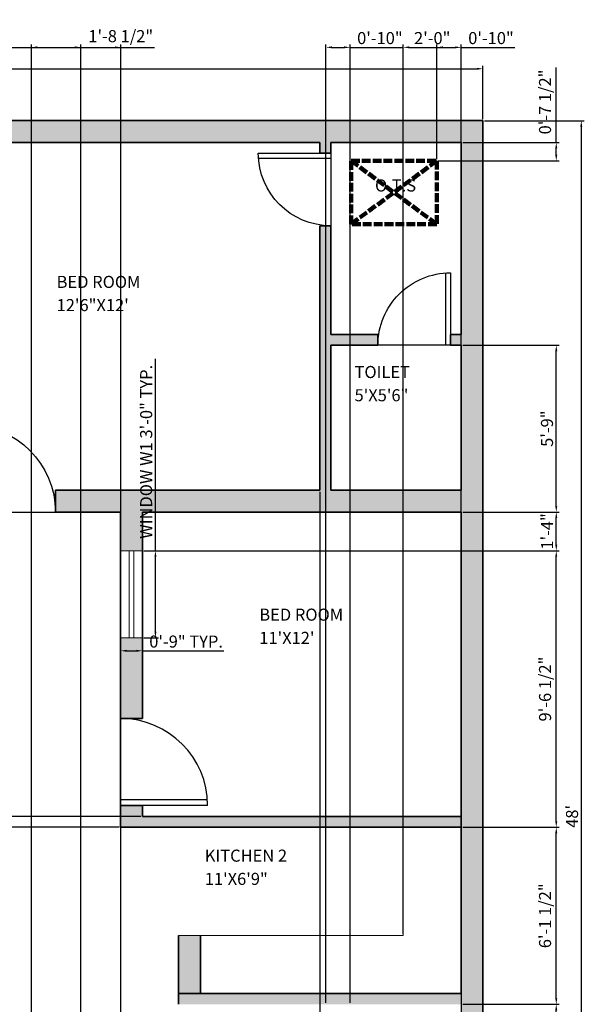
# Model space of a CAD drawing. Units: inches. Extents: x 2263 to 2802, y 2658 to 3310.
# Tile 3 of 3: x 2569 to 2802, y 2902 to 3310. Entities that reach past the tile are written whole.
import ezdxf

# ---------------------------------------------------------------- set-up
doc = ezdxf.new("R2010")
doc.units = ezdxf.units.IN
doc.header["$LTSCALE"] = 0.3
doc.linetypes.add('ACAD_ISO02W100', pattern=[15, 12, -3])
for name, color, linetype, lineweight in [('A-ANNO-DIMS', 2, 'Continuous', 18), ('A-AREA-IDEN', 7, 'Continuous', 18), ('A-DOOR', 3, 'Continuous', 25), ('A-FLOR-FIXT', 8, 'Continuous', 18), ('A-GLAZ', 4, 'Continuous', 18), ('A-ROOF-OVHD', 7, 'ACAD_ISO02W100', 100), ('A-WALL', 7, 'Continuous', 35)]:
    doc.layers.add(name, color=color, linetype=linetype, lineweight=lineweight)
doc.layers.add('A-WALL-PATT', color=18, linetype='Continuous', lineweight=13, true_color=0x000000)
doc.styles.get("Standard").update_dxf_attribs({"font": 'calibri.ttf', "height": 5})
doc.dimstyles.new('ISO-25', dxfattribs={"dimtxt": 5, "dimasz": 2.5, "dimexe": 1.25, "dimexo": 0.625, "dimtad": 1, "dimlunit": 3, "dimtxsty": 'Standard', "dimcen": 2.5, "dimadec": 0, "dimazin": 0, "dimtfac": 1, "dimtmove": 0, "dimatfit": 3, "dimfxl": 1, "dimarcsym": 0})

# ---------------------------------------------------------------- blocks, each defined once
blk = doc.blocks.new('*D1')
at = {"layer": 'A-ANNO-DIMS', "color": 0, "lineweight": -2, "transparency": 16777216}
for p, q in [((2304.41, 3268.9), (2304.41, 3291.01)), ((2306.91, 3289.76), (2757.91, 3289.76)), ((2760.41, 3268.9), (2760.41, 3291.01))]:
    blk.add_line(p, q, dxfattribs=at)
at = {"layer": 'A-ANNO-DIMS', "color": 0, "lineweight": -3, "transparency": 16777216}
for points in [[(2306.91, 3290.17), (2306.91, 3289.34), (2304.41, 3289.76)], [(2757.91, 3290.17), (2757.91, 3289.34), (2760.41, 3289.76)]]:
    blk.add_solid(points, dxfattribs=at)
at = {"layer": 'Defpoints', "color": 0, "lineweight": -3, "transparency": 16777216}
for p in [(2760.41, 3289.76), (2304.41, 3268.27), (2760.41, 3268.27)]:
    blk.add_point(p, dxfattribs=at)
at = {"layer": 'A-ANNO-DIMS', "color": 0, "transparency": 16777216, "insert": (2532.41, 3292.94), "char_height": 5, "attachment_point": 5}
blk.add_mtext("38'", dxfattribs=at)
blk = doc.blocks.new('*D2')
at = {"layer": 'A-ANNO-DIMS', "color": 0, "lineweight": -2, "transparency": 16777216}
for p, q in [((2761.03, 3268.27), (2802.38, 3268.27)), ((2801.13, 3265.77), (2801.13, 2694.77)), ((2761.03, 2692.27), (2802.38, 2692.27))]:
    blk.add_line(p, q, dxfattribs=at)
at = {"layer": 'A-ANNO-DIMS', "color": 0, "lineweight": -3, "transparency": 16777216}
for points in [[(2800.71, 3265.77), (2801.54, 3265.77), (2801.13, 3268.27)], [(2800.71, 2694.77), (2801.54, 2694.77), (2801.13, 2692.27)]]:
    blk.add_solid(points, dxfattribs=at)
at = {"layer": 'Defpoints', "color": 0, "lineweight": -3, "transparency": 16777216}
for p in [(2760.41, 3268.27), (2760.41, 2692.27), (2801.13, 2692.27)]:
    blk.add_point(p, dxfattribs=at)
at = {"layer": 'A-ANNO-DIMS', "color": 0, "transparency": 16777216, "insert": (2797.94, 2980.27), "char_height": 5, "attachment_point": 5, "rotation": 90}
blk.add_mtext("48'", dxfattribs=at)
blk = doc.blocks.new('DOOR-SWING-36')
for p, q in [((0, 0), (0, 36)), ((35.92, 2.4), (0, 2.4)), ((36, 0), (0, 0))]:
    blk.add_line(p, q)
blk.add_arc((0, 0), 36, 0, 90)
blk = doc.blocks.new('DOOR-SWING-30')
for p, q in [((30, 0), (0, 0)), ((0, 0), (0, -30)), ((29.93, -2), (0, -2))]:
    blk.add_line(p, q)
blk.add_arc((0, 0), 30, 270, 0)
blk = doc.blocks.new('WIN-36')
for p, q in [((0, 36), (-9, 36)), ((-9, 36), (-9, 0)), ((-5.5, 0), (-5.5, 36)), ((-3.5, 0), (-3.5, 36)), ((0, 0), (0, 36)), ((-9, 0), (0, 0))]:
    blk.add_line(p, q)
blk = doc.blocks.new('OPEN-TO-SKY')
for p, q in [((0, 0), (35.52, 0)), ((0, -26.28), (0, 0)), ((0, 0), (35.52, -26.28)), ((35.52, 0), (0, -26.28)), ((35.52, 0), (35.52, -26.28)), ((35.52, -26.28), (0, -26.28))]:
    blk.add_line(p, q)
blk = doc.blocks.new('*D13')
at = {"layer": 'A-ANNO-DIMS', "color": 0, "lineweight": -2, "transparency": 16777216}
for p, q in [((2624.81, 3090.22), (2624.81, 3169.67)), ((2620.03, 3090.22), (2626.06, 3090.22)), ((2624.81, 3056.72), (2624.81, 3087.72)), ((2620.03, 3054.22), (2626.06, 3054.22))]:
    blk.add_line(p, q, dxfattribs=at)
at = {"layer": 'A-ANNO-DIMS', "color": 0, "lineweight": -3, "transparency": 16777216}
for points in [[(2624.39, 3087.72), (2625.23, 3087.72), (2624.81, 3090.22)], [(2624.39, 3056.72), (2625.23, 3056.72), (2624.81, 3054.22)]]:
    blk.add_solid(points, dxfattribs=at)
at = {"layer": 'Defpoints', "color": 0, "lineweight": -3, "transparency": 16777216}
for p in [(2619.41, 3090.22), (2624.81, 3090.22), (2619.41, 3054.22)]:
    blk.add_point(p, dxfattribs=at)
at = {"layer": 'A-ANNO-DIMS', "color": 0, "transparency": 16777216, "insert": (2621.62, 3131.19), "char_height": 5, "attachment_point": 5, "rotation": 90}
blk.add_mtext('WINDOW W1 3\'-0" TYP.', dxfattribs=at)
blk = doc.blocks.new('*D14')
at = {"layer": 'A-ANNO-DIMS', "color": 0, "lineweight": -2, "transparency": 16777216}
for p, q in [((2610.41, 3053.59), (2610.41, 3047.57)), ((2619.41, 3053.59), (2619.41, 3047.57)), ((2612.91, 3048.82), (2616.91, 3048.82)), ((2619.41, 3048.82), (2653.11, 3048.82))]:
    blk.add_line(p, q, dxfattribs=at)
at = {"layer": 'A-ANNO-DIMS', "color": 0, "lineweight": -3, "transparency": 16777216}
for points in [[(2612.91, 3049.23), (2612.91, 3048.4), (2610.41, 3048.82)], [(2616.91, 3049.23), (2616.91, 3048.4), (2619.41, 3048.82)]]:
    blk.add_solid(points, dxfattribs=at)
at = {"layer": 'Defpoints', "color": 0, "lineweight": -3, "transparency": 16777216}
for p in [(2610.41, 3054.22), (2619.41, 3054.22), (2619.41, 3048.82)]:
    blk.add_point(p, dxfattribs=at)
at = {"layer": 'A-ANNO-DIMS', "color": 0, "transparency": 16777216, "insert": (2637.51, 3052), "char_height": 5, "attachment_point": 5}
blk.add_mtext('0\'-9" TYP.', dxfattribs=at)
blk = doc.blocks.new('*D30')
at = {"layer": 'A-ANNO-DIMS', "color": 0, "lineweight": -2, "transparency": 16777216}
for p, q in [((2573.46, 2770.9), (2573.46, 3299.87)), ((2575.96, 3298.62), (2591.41, 3298.62)), ((2593.91, 2770.9), (2593.91, 3299.87)), ((2593.91, 3298.62), (2624.49, 3298.62))]:
    blk.add_line(p, q, dxfattribs=at)
at = {"layer": 'A-ANNO-DIMS', "color": 0, "lineweight": -3, "transparency": 16777216}
for points in [[(2575.96, 3299.04), (2575.96, 3298.21), (2573.46, 3298.62)], [(2591.41, 3299.04), (2591.41, 3298.21), (2593.91, 3298.62)]]:
    blk.add_solid(points, dxfattribs=at)
at = {"layer": 'Defpoints', "color": 0, "lineweight": -3, "transparency": 16777216}
for p in [(2593.91, 3298.62), (2573.46, 2770.27), (2593.91, 2770.27)]:
    blk.add_point(p, dxfattribs=at)
at = {"layer": 'A-ANNO-DIMS', "color": 0, "transparency": 16777216, "insert": (2610.45, 3302.61), "char_height": 5, "attachment_point": 5}
blk.add_mtext('1\'-8 1/2"', dxfattribs=at)
blk = doc.blocks.new('*D33')
at = {"layer": 'A-ANNO-DIMS', "color": 0, "lineweight": -2, "transparency": 16777216}
for p, q in [((2695.41, 2903.1), (2695.41, 3299.87)), ((2697.91, 3298.62), (2702.91, 3298.62)), ((2705.41, 2903.1), (2705.41, 3299.87)), ((2705.41, 3298.62), (2727.57, 3298.62))]:
    blk.add_line(p, q, dxfattribs=at)
at = {"layer": 'A-ANNO-DIMS', "color": 0, "lineweight": -3, "transparency": 16777216}
for points in [[(2697.91, 3299.04), (2697.91, 3298.21), (2695.41, 3298.62)], [(2702.91, 3299.04), (2702.91, 3298.21), (2705.41, 3298.62)]]:
    blk.add_solid(points, dxfattribs=at)
at = {"layer": 'Defpoints', "color": 0, "lineweight": -3, "transparency": 16777216}
for p in [(2705.41, 3298.62), (2695.41, 2902.48), (2705.41, 2902.48)]:
    blk.add_point(p, dxfattribs=at)
at = {"layer": 'A-ANNO-DIMS', "color": 0, "transparency": 16777216, "insert": (2717.74, 3301.81), "char_height": 5, "attachment_point": 5}
blk.add_mtext('0\'-10"', dxfattribs=at)
blk = doc.blocks.new('*D34')
at = {"layer": 'A-ANNO-DIMS', "color": 0, "lineweight": -2, "transparency": 16777216}
for p, q in [((2727.41, 2931.6), (2727.41, 3299.87)), ((2729.91, 3298.62), (2748.91, 3298.62)), ((2751.41, 2907.6), (2751.41, 3299.87))]:
    blk.add_line(p, q, dxfattribs=at)
at = {"layer": 'A-ANNO-DIMS', "color": 0, "lineweight": -3, "transparency": 16777216}
for points in [[(2729.91, 3299.04), (2729.91, 3298.21), (2727.41, 3298.62)], [(2748.91, 3299.04), (2748.91, 3298.21), (2751.41, 3298.62)]]:
    blk.add_solid(points, dxfattribs=at)
at = {"layer": 'Defpoints', "color": 0, "lineweight": -3, "transparency": 16777216}
for p in [(2751.41, 3298.62), (2727.41, 2930.98), (2751.41, 2906.98)]:
    blk.add_point(p, dxfattribs=at)
at = {"layer": 'A-ANNO-DIMS', "color": 0, "transparency": 16777216, "insert": (2739.41, 3301.81), "char_height": 5, "attachment_point": 5}
blk.add_mtext('2\'-0"', dxfattribs=at)
blk = doc.blocks.new('*D35')
at = {"layer": 'A-ANNO-DIMS', "color": 0, "lineweight": -2, "transparency": 16777216}
for p, q in [((2274.06, 2982.77), (2274.06, 3013.75)), ((2618.78, 2980.27), (2272.81, 2980.27)), ((2274.06, 2975.77), (2274.06, 2980.27)), ((2609.78, 2975.77), (2272.81, 2975.77)), ((2274.06, 2973.27), (2274.06, 2970.77))]:
    blk.add_line(p, q, dxfattribs=at)
at = {"layer": 'A-ANNO-DIMS', "color": 0, "lineweight": -3, "transparency": 16777216}
for points in [[(2273.64, 2982.77), (2274.48, 2982.77), (2274.06, 2980.27)], [(2273.64, 2973.27), (2274.48, 2973.27), (2274.06, 2975.77)]]:
    blk.add_solid(points, dxfattribs=at)
at = {"layer": 'Defpoints', "color": 0, "lineweight": -3, "transparency": 16777216}
for p in [(2274.06, 2980.27), (2619.41, 2980.27), (2610.41, 2975.77)]:
    blk.add_point(p, dxfattribs=at)
at = {"layer": 'A-ANNO-DIMS', "color": 0, "transparency": 16777216, "insert": (2270.07, 2999.51), "char_height": 5, "attachment_point": 5, "rotation": 90}
blk.add_mtext('0\'-4 1/2"', dxfattribs=at)
blk = doc.blocks.new('*D37')
at = {"layer": 'A-ANNO-DIMS', "color": 0, "lineweight": -2, "transparency": 16777216}
for p, q in [((2752.03, 2902.48), (2792.01, 2902.48)), ((2790.76, 2790.6), (2790.76, 2899.98)), ((2752.03, 2788.1), (2792.01, 2788.1))]:
    blk.add_line(p, q, dxfattribs=at)
at = {"layer": 'A-ANNO-DIMS', "color": 0, "lineweight": -3, "transparency": 16777216}
for points in [[(2790.34, 2899.98), (2791.18, 2899.98), (2790.76, 2902.48)], [(2790.34, 2790.6), (2791.18, 2790.6), (2790.76, 2788.1)]]:
    blk.add_solid(points, dxfattribs=at)
at = {"layer": 'Defpoints', "color": 0, "lineweight": -3, "transparency": 16777216}
for p in [(2751.41, 2902.48), (2790.76, 2902.48), (2751.41, 2788.1)]:
    blk.add_point(p, dxfattribs=at)
at = {"layer": 'A-ANNO-DIMS', "color": 0, "transparency": 16777216, "insert": (2786.77, 2845.29), "char_height": 5, "attachment_point": 5, "rotation": 90}
blk.add_mtext('9\'-6 1/2"', dxfattribs=at)
blk = doc.blocks.new('*D38')
at = {"layer": 'A-ANNO-DIMS', "color": 0, "lineweight": -2, "transparency": 16777216}
for p, q in [((2752.03, 2975.77), (2792.01, 2975.77)), ((2790.76, 2904.98), (2790.76, 2973.27)), ((2752.03, 2902.48), (2792.01, 2902.48))]:
    blk.add_line(p, q, dxfattribs=at)
at = {"layer": 'A-ANNO-DIMS', "color": 0, "lineweight": -3, "transparency": 16777216}
for points in [[(2790.34, 2973.27), (2791.18, 2973.27), (2790.76, 2975.77)], [(2790.34, 2904.98), (2791.18, 2904.98), (2790.76, 2902.48)]]:
    blk.add_solid(points, dxfattribs=at)
at = {"layer": 'Defpoints', "color": 0, "lineweight": -3, "transparency": 16777216}
for p in [(2751.41, 2975.77), (2790.76, 2975.77), (2751.41, 2902.48)]:
    blk.add_point(p, dxfattribs=at)
at = {"layer": 'A-ANNO-DIMS', "color": 0, "transparency": 16777216, "insert": (2786.77, 2939.12), "char_height": 5, "attachment_point": 5, "rotation": 90}
blk.add_mtext('6\'-1 1/2"', dxfattribs=at)
blk = doc.blocks.new('*D39')
at = {"layer": 'A-ANNO-DIMS', "color": 0, "lineweight": -2, "transparency": 16777216}
for p, q in [((2620.03, 3090.22), (2792.01, 3090.22)), ((2790.76, 2978.27), (2790.76, 3087.72)), ((2752.03, 2975.77), (2792.01, 2975.77))]:
    blk.add_line(p, q, dxfattribs=at)
at = {"layer": 'A-ANNO-DIMS', "color": 0, "lineweight": -3, "transparency": 16777216}
for points in [[(2790.34, 3087.72), (2791.18, 3087.72), (2790.76, 3090.22)], [(2790.34, 2978.27), (2791.18, 2978.27), (2790.76, 2975.77)]]:
    blk.add_solid(points, dxfattribs=at)
at = {"layer": 'Defpoints', "color": 0, "lineweight": -3, "transparency": 16777216}
for p in [(2619.41, 3090.22), (2790.76, 3090.22), (2751.41, 2975.77)]:
    blk.add_point(p, dxfattribs=at)
at = {"layer": 'A-ANNO-DIMS', "color": 0, "transparency": 16777216, "insert": (2786.77, 3032.99), "char_height": 5, "attachment_point": 5, "rotation": 90}
blk.add_mtext('9\'-6 1/2"', dxfattribs=at)
blk = doc.blocks.new('*D40')
at = {"layer": 'A-ANNO-DIMS', "color": 0, "lineweight": -2, "transparency": 16777216}
for p, q in [((2752.03, 3106.27), (2792.01, 3106.27)), ((2790.76, 3092.72), (2790.76, 3103.77)), ((2620.03, 3090.22), (2792.01, 3090.22))]:
    blk.add_line(p, q, dxfattribs=at)
at = {"layer": 'A-ANNO-DIMS', "color": 0, "lineweight": -3, "transparency": 16777216}
for points in [[(2790.34, 3103.77), (2791.18, 3103.77), (2790.76, 3106.27)], [(2790.34, 3092.72), (2791.18, 3092.72), (2790.76, 3090.22)]]:
    blk.add_solid(points, dxfattribs=at)
at = {"layer": 'Defpoints', "color": 0, "lineweight": -3, "transparency": 16777216}
for p in [(2751.41, 3106.27), (2790.76, 3106.27), (2619.41, 3090.22)]:
    blk.add_point(p, dxfattribs=at)
at = {"layer": 'A-ANNO-DIMS', "color": 0, "transparency": 16777216, "insert": (2787.62, 3098.24), "char_height": 5, "attachment_point": 5, "rotation": 90}
blk.add_mtext('1\'-4"', dxfattribs=at)
blk = doc.blocks.new('*D41')
at = {"layer": 'A-ANNO-DIMS', "color": 0, "lineweight": -2, "transparency": 16777216}
for p, q in [((2752.03, 3175.27), (2792.01, 3175.27)), ((2790.76, 3108.77), (2790.76, 3172.77)), ((2752.03, 3106.27), (2792.01, 3106.27))]:
    blk.add_line(p, q, dxfattribs=at)
at = {"layer": 'A-ANNO-DIMS', "color": 0, "lineweight": -3, "transparency": 16777216}
for points in [[(2790.34, 3172.77), (2791.18, 3172.77), (2790.76, 3175.27)], [(2790.34, 3108.77), (2791.18, 3108.77), (2790.76, 3106.27)]]:
    blk.add_solid(points, dxfattribs=at)
at = {"layer": 'Defpoints', "color": 0, "lineweight": -3, "transparency": 16777216}
for p in [(2751.41, 3175.27), (2790.76, 3175.27), (2751.41, 3106.27)]:
    blk.add_point(p, dxfattribs=at)
at = {"layer": 'A-ANNO-DIMS', "color": 0, "transparency": 16777216, "insert": (2787.57, 3140.77), "char_height": 5, "attachment_point": 5, "rotation": 90}
blk.add_mtext('5\'-9"', dxfattribs=at)
blk = doc.blocks.new('*D42')
at = {"layer": 'A-ANNO-DIMS', "color": 0, "lineweight": -2, "transparency": 16777216}
for p, q in [((2468.29, 2867.1), (2468.29, 3299.87)), ((2470.79, 3298.62), (2608, 3298.62)), ((2610.5, 2867.1), (2610.5, 3299.87))]:
    blk.add_line(p, q, dxfattribs=at)
at = {"layer": 'A-ANNO-DIMS', "color": 0, "lineweight": -3, "transparency": 16777216}
for points in [[(2470.79, 3299.04), (2470.79, 3298.21), (2468.29, 3298.62)], [(2608, 3299.04), (2608, 3298.21), (2610.5, 3298.62)]]:
    blk.add_solid(points, dxfattribs=at)
at = {"layer": 'Defpoints', "color": 0, "lineweight": -3, "transparency": 16777216}
for p in [(2610.5, 3298.62), (2468.29, 2866.48), (2610.5, 2866.48)]:
    blk.add_point(p, dxfattribs=at)
at = {"layer": 'A-ANNO-DIMS', "color": 0, "transparency": 16777216, "insert": (2539.4, 3301.81), "char_height": 5, "attachment_point": 5}
blk.add_mtext('11\'-10"', dxfattribs=at)
blk = doc.blocks.new('*D44')
at = {"layer": 'A-ANNO-DIMS', "color": 0, "lineweight": -2, "transparency": 16777216}
for p, q in [((2692.91, 3114.65), (2692.91, 2660.67)), ((2751.41, 3105.65), (2751.41, 2660.67)), ((2695.41, 2661.92), (2748.91, 2661.92))]:
    blk.add_line(p, q, dxfattribs=at)
at = {"layer": 'A-ANNO-DIMS', "color": 0, "lineweight": -3, "transparency": 16777216}
for points in [[(2695.41, 2662.34), (2695.41, 2661.51), (2692.91, 2661.92)], [(2748.91, 2662.34), (2748.91, 2661.51), (2751.41, 2661.92)]]:
    blk.add_solid(points, dxfattribs=at)
at = {"layer": 'Defpoints', "color": 0, "lineweight": -3, "transparency": 16777216}
for p in [(2692.91, 3115.27), (2751.41, 3106.27), (2751.41, 2661.92)]:
    blk.add_point(p, dxfattribs=at)
at = {"layer": 'A-ANNO-DIMS', "color": 0, "transparency": 16777216, "insert": (2722.16, 2665.91), "char_height": 5, "attachment_point": 5}
blk.add_mtext('4\'-10 1/2"', dxfattribs=at)
blk = doc.blocks.new('*D45')
at = {"layer": 'A-ANNO-DIMS', "color": 0, "lineweight": -2, "transparency": 16777216}
for p, q in [((2741.31, 3252.32), (2741.31, 3299.87)), ((2743.81, 3298.62), (2748.91, 3298.62)), ((2751.41, 3259.9), (2751.41, 3299.87)), ((2751.41, 3298.62), (2773.57, 3298.62))]:
    blk.add_line(p, q, dxfattribs=at)
at = {"layer": 'A-ANNO-DIMS', "color": 0, "lineweight": -3, "transparency": 16777216}
for points in [[(2743.81, 3299.04), (2743.81, 3298.21), (2741.31, 3298.62)], [(2748.91, 3299.04), (2748.91, 3298.21), (2751.41, 3298.62)]]:
    blk.add_solid(points, dxfattribs=at)
at = {"layer": 'Defpoints', "color": 0, "lineweight": -3, "transparency": 16777216}
for p in [(2751.41, 3298.62), (2751.41, 3259.27), (2741.31, 3251.69)]:
    blk.add_point(p, dxfattribs=at)
at = {"layer": 'A-ANNO-DIMS', "color": 0, "transparency": 16777216, "insert": (2763.74, 3301.81), "char_height": 5, "attachment_point": 5}
blk.add_mtext('0\'-10"', dxfattribs=at)
blk = doc.blocks.new('*D46')
at = {"layer": 'A-ANNO-DIMS', "color": 0, "lineweight": -2, "transparency": 16777216}
for p, q in [((2790.76, 3259.27), (2790.76, 3290.25)), ((2752.03, 3259.27), (2792.01, 3259.27)), ((2790.76, 3254.19), (2790.76, 3256.77)), ((2741.93, 3251.69), (2792.01, 3251.69))]:
    blk.add_line(p, q, dxfattribs=at)
at = {"layer": 'A-ANNO-DIMS', "color": 0, "lineweight": -3, "transparency": 16777216}
for points in [[(2790.34, 3256.77), (2791.18, 3256.77), (2790.76, 3259.27)], [(2790.34, 3254.19), (2791.18, 3254.19), (2790.76, 3251.69)]]:
    blk.add_solid(points, dxfattribs=at)
at = {"layer": 'Defpoints', "color": 0, "lineweight": -3, "transparency": 16777216}
for p in [(2751.41, 3259.27), (2790.76, 3259.27), (2741.31, 3251.69)]:
    blk.add_point(p, dxfattribs=at)
at = {"layer": 'A-ANNO-DIMS', "color": 0, "transparency": 16777216, "insert": (2786.77, 3276.01), "char_height": 5, "attachment_point": 5, "rotation": 90}
blk.add_mtext('0\'-7 1/2"', dxfattribs=at)

msp = doc.modelspace()

# ---------------------------------------------------------------- hatches: boundary and pattern name
at = {"layer": 'A-WALL-PATT'}
h = msp.add_hatch(color=256, dxfattribs=at)
h.dxf.hatch_style = 1
h.paths.add_polyline_path([(2454.409, 2984.773), (2445.409, 2984.773), (2445.409, 2980.273), (2313.409, 2980.273), (2313.409, 3019.273), (2304.409, 3019.273), (2304.409, 2959.375), (2313.409, 2959.375), (2313.409, 2975.773), (2454.409, 2975.773)], flags=17)
h.paths.add_polyline_path([(2313.409, 2902.477), (2454.409, 2902.477), (2454.409, 2906.977), (2313.409, 2906.977), (2313.409, 2923.375), (2304.409, 2923.375), (2304.409, 2860.375), (2313.409, 2860.375)], flags=17)
h.paths.add_polyline_path([(2313.409, 2812.375), (2304.409, 2812.375), (2304.409, 2692.273), (2334.409, 2692.273), (2334.409, 2701.273), (2313.409, 2701.273), (2313.409, 2761.273), (2379.409, 2761.273), (2379.409, 2735.773), (2383.909, 2735.773), (2383.909, 2761.273), (2396.251, 2761.273), (2396.251, 2770.273), (2313.409, 2770.273)], flags=17)
h.paths.add_polyline_path([(2760.409, 3268.273), (2304.409, 3268.273), (2304.409, 3157.273), (2313.409, 3157.273), (2313.409, 3175.273), (2317.909, 3175.273), (2317.909, 3179.773), (2313.409, 3179.773), (2313.409, 3259.273), (2379.409, 3259.273), (2379.409, 3254.773), (2383.909, 3254.773), (2383.909, 3259.273), (2533.909, 3259.273), (2533.909, 3115.273), (2529.409, 3115.273), (2529.409, 3106.273), (2547.409, 3106.273), (2547.409, 3115.273), (2542.909, 3115.273), (2542.909, 3259.273), (2692.909, 3259.273), (2692.909, 3254.773), (2697.409, 3254.773), (2697.409, 3259.273), (2751.409, 3259.273), (2751.409, 3179.773), (2746.909, 3179.773), (2746.909, 3175.273), (2751.409, 3175.273), (2751.409, 3115.273), (2697.409, 3115.273), (2697.409, 3175.273), (2716.909, 3175.273), (2716.909, 3179.773), (2697.409, 3179.773), (2697.409, 3224.773), (2692.909, 3224.773), (2692.909, 3115.273), (2583.409, 3115.273), (2583.409, 3106.273), (2610.409, 3106.273), (2610.409, 3090.217), (2619.409, 3090.217), (2619.409, 3106.273), (2751.409, 3106.273), (2751.409, 2980.273), (2619.409, 2980.273), (2619.409, 2984.773), (2610.409, 2984.773), (2610.409, 2975.773), (2751.409, 2975.773), (2751.409, 2906.977), (2634.409, 2906.977), (2634.409, 2902.477), (2670.409, 2902.477), (2751.409, 2902.477), (2751.409, 2701.273), (2383.909, 2701.273), (2383.909, 2705.773), (2379.409, 2705.773), (2379.409, 2701.273), (2358.409, 2701.273), (2358.409, 2692.273), (2760.409, 2692.273)])
h.paths.add_polyline_path([(2501.459, 2770.273), (2454.409, 2770.273), (2454.409, 2857.477), (2468.293, 2857.477), (2468.293, 2866.477), (2445.409, 2866.477), (2445.409, 2770.273), (2432.251, 2770.273), (2432.251, 2761.273), (2501.459, 2761.273)], flags=17)
h.paths.add_polyline_path([(2593.909, 2770.273), (2573.459, 2770.273), (2573.459, 2761.273), (2593.909, 2761.273)], flags=17)
h.paths.add_polyline_path([(2643.409, 2866.477), (2610.501, 2866.477), (2610.501, 2857.477), (2634.409, 2857.477), (2634.409, 2770.273), (2629.909, 2770.273), (2629.909, 2761.273), (2643.409, 2761.273)], flags=17)
h.paths.add_polyline_path([(2643.409, 2930.977), (2634.409, 2930.977), (2634.409, 2906.977), (2643.409, 2906.977)], flags=17)
h.paths.add_polyline_path([(2454.409, 2930.977), (2445.409, 2930.977), (2445.409, 2906.977), (2454.409, 2906.977)], flags=17)
h.paths.add_polyline_path([(2454.409, 3106.273), (2493.409, 3106.273), (2493.409, 3115.273), (2383.909, 3115.273), (2383.909, 3224.773), (2379.409, 3224.773), (2379.409, 3179.773), (2347.909, 3179.773), (2347.909, 3175.273), (2379.409, 3175.273), (2379.409, 3115.273), (2313.409, 3115.273), (2313.409, 3133.273), (2304.409, 3133.273), (2304.409, 3067.273), (2313.409, 3067.273), (2313.409, 3106.273), (2445.409, 3106.273), (2445.409, 3020.773), (2454.409, 3020.773)], flags=17)
h.paths.add_polyline_path([(2619.409, 3054.217), (2610.409, 3054.217), (2610.409, 3020.773), (2619.409, 3020.773)], flags=17)

# ---------------------------------------------------------------- linework, layer by layer
at = {"layer": 'A-FLOR-FIXT'}
for p in [(2727.409, 2975.773), (2634.409, 2930.977)]:
    msp.add_line(p, (2727.409, 2930.977), dxfattribs=at)
at = {"layer": 'A-WALL'}
for p, q in [((2304.409, 3268.273), (2760.409, 3268.273)), ((2760.409, 3268.273), (2760.409, 2692.273)), ((2542.909, 3259.273), (2692.909, 3259.273)), ((2692.909, 3254.773), (2692.909, 3259.273)), ((2697.409, 3259.273), (2751.409, 3259.273)), ((2697.409, 3254.773), (2697.409, 3259.273)), ((2751.409, 3259.273), (2751.409, 3179.773)), ((2692.909, 3254.773), (2697.409, 3254.773)), ((2692.909, 3115.273), (2692.909, 3224.773)), ((2692.909, 3224.773), (2697.409, 3224.773)), ((2697.409, 3179.773), (2697.409, 3224.773)), ((2697.409, 3179.773), (2716.909, 3179.773)), ((2716.909, 3175.273), (2716.909, 3179.773)), ((2746.909, 3175.273), (2746.909, 3179.773)), ((2746.909, 3179.773), (2751.409, 3179.773)), ((2697.409, 3115.273), (2697.409, 3175.273)), ((2697.409, 3175.273), (2716.909, 3175.273)), ((2746.909, 3175.273), (2751.409, 3175.273)), ((2751.409, 3175.273), (2751.409, 3115.273)), ((2583.409, 3115.273), (2583.409, 3106.273)), ((2583.409, 3115.273), (2692.909, 3115.273)), ((2697.409, 3115.273), (2751.409, 3115.273)), ((2583.409, 3106.273), (2610.409, 3106.273)), ((2610.409, 3106.273), (2610.409, 3020.773)), ((2619.409, 3106.273), (2619.409, 3020.773)), ((2619.409, 3106.273), (2751.409, 3106.273)), ((2751.409, 3106.273), (2751.409, 2980.273)), ((2619.409, 3020.773), (2610.409, 3020.773)), ((2619.409, 2984.773), (2610.409, 2984.773)), ((2610.409, 2984.773), (2610.409, 2975.773)), ((2619.409, 2984.773), (2619.409, 2980.273)), ((2619.409, 2980.273), (2751.409, 2980.273)), ((2610.409, 2975.773), (2751.409, 2975.773)), ((2751.409, 2975.773), (2751.409, 2906.977)), ((2634.409, 2930.977), (2634.409, 2906.977)), ((2643.409, 2930.977), (2643.409, 2906.977)), ((2634.409, 2906.977), (2634.409, 2902.477)), ((2634.409, 2906.977), (2751.409, 2906.977))]:
    msp.add_line(p, q, dxfattribs=at)

# ---------------------------------------------------------------- block references
at = {"layer": 'A-DOOR', "extrusion": (0, 0, -1), "zscale": -1}
msp.add_blockref('DOOR-SWING-30', (-2697.409, 3254.773), dxfattribs=at)
for name, p, rotation in [('DOOR-SWING-30', (-2746.909, 3175.273), 90.00000000000426), ('DOOR-SWING-36', (-2547.409, 3106.273), 89.99999999999883)]:
    msp.add_blockref(name, p, dxfattribs=dict(at, rotation=rotation))
at = {"layer": 'A-DOOR'}
msp.add_blockref('DOOR-SWING-36', (2610.409, 2984.773), dxfattribs=at)
at = {"layer": 'A-GLAZ'}
msp.add_blockref('WIN-36', (2619.409, 3054.217), dxfattribs=at)
at = {"layer": 'A-ROOF-OVHD'}
msp.add_blockref('OPEN-TO-SKY', (2705.787, 3251.693), dxfattribs=at)

# ---------------------------------------------------------------- texts
at = {"layer": 'A-AREA-IDEN'}
for s, p in [('O.T.S', (2715.711, 3238.934)), ('BED ROOM', (2583.901, 3199.027)), ('12\'6"X12\'', (2583.901, 3189.412)), ('TOILET', (2707.245, 3161.725)), ('5\'X5\'6"', (2707.245, 3152.109)), ('BED ROOM', (2667.821, 3061.28)), ("11'X12'", (2667.821, 3051.665)), ('KITCHEN 2', (2645.249, 2961.515)), ('11\'X6\'9"', (2645.249, 2951.9))]:
    msp.add_text(s, height=5, dxfattribs=at).set_placement(p)

# ---------------------------------------------------------------- dimensions: what is measured, and where the dimension line sits
at = {"layer": 'A-ANNO-DIMS'}
for base, p1, p2, override, picture, middle in [((2593.9094, 3298.6226), (2573.459, 2770.2726), (2593.9094, 2770.2726), {"dimdec": 1, "dimlfac": 1, "dimrnd": 0, "dimzin": 1, "dimdsep": 46, "dimlunit": 4, "dimfrac": 2}, '*D30', (2610.4517, 3302.6149)), ((2610.501, 3298.623), (2468.293, 2866.477), (2610.501, 2866.477), {"dimdec": 1, "dimlfac": 1, "dimrnd": 0, "dimzin": 1, "dimdsep": 46, "dimlunit": 4, "dimfrac": 2}, '*D42', (2539.397, 3301.809)), ((2705.409, 3298.623), (2695.409, 2902.477), (2705.409, 2902.477), {"dimdec": 1, "dimlfac": 1, "dimrnd": 0, "dimzin": 1, "dimdsep": 46, "dimlunit": 4, "dimfrac": 2}, '*D33', (2717.74, 3301.809)), ((2751.409, 3298.623), (2727.409, 2930.977), (2751.409, 2906.977), {"dimdec": 1, "dimlfac": 1, "dimrnd": 0, "dimzin": 1, "dimdsep": 46, "dimlunit": 4, "dimfrac": 2}, '*D34', (2739.409, 3301.809)), ((2751.409, 3298.623), (2741.305, 3251.693), (2751.409, 3259.273), {"dimdec": 1, "dimlfac": 1, "dimrnd": 0, "dimzin": 1, "dimdsep": 46, "dimlunit": 4, "dimfrac": 2}, '*D45', (2763.74, 3301.809)), ((2760.409, 3289.757), (2304.409, 3268.273), (2760.409, 3268.273), {"dimclrd": 0, "dimclre": 0, "dimclrt": 0}, '*D1', (2532.409, 3292.944)), ((2751.409, 2661.923), (2692.909, 3115.273), (2751.409, 3106.273), {"dimdec": 1, "dimlfac": 1, "dimrnd": 0, "dimzin": 1, "dimdsep": 46, "dimlunit": 4, "dimfrac": 2}, '*D44', (2722.159, 2665.915))]:
    dim = msp.add_linear_dim(base=base, p1=p1, p2=p2, dimstyle='ISO-25', override=override, dxfattribs=at)
    dim.commit()
    dim.dimension.update_dxf_attribs({"geometry": picture, "text_midpoint": middle})
for base, p1, p2, override, picture, middle in [((2790.759, 3259.273), (2741.305, 3251.693), (2751.409, 3259.273), {"dimdec": 1, "dimlfac": 1, "dimrnd": 0, "dimzin": 1, "dimdsep": 46, "dimlunit": 4, "dimfrac": 2}, '*D46', (2786.767, 3276.011)), ((2801.125, 2692.273), (2760.409, 3268.273), (2760.409, 2692.273), {"dimclrd": 0, "dimclre": 0, "dimclrt": 0}, '*D2', (2797.939, 2980.273)), ((2790.759, 3175.273), (2751.409, 3106.273), (2751.409, 3175.273), {"dimdec": 1, "dimlfac": 1, "dimrnd": 0, "dimzin": 1, "dimdsep": 46, "dimlunit": 4, "dimfrac": 2}, '*D41', (2787.573, 3140.773)), ((2790.759, 3106.273), (2619.409, 3090.217), (2751.409, 3106.273), {"dimdec": 1, "dimlfac": 1, "dimrnd": 0, "dimzin": 1, "dimdsep": 46, "dimlunit": 4, "dimfrac": 2}, '*D40', (2787.617, 3098.245)), ((2790.759, 3090.217), (2751.409, 2975.773), (2619.409, 3090.217), {"dimdec": 1, "dimlfac": 1, "dimrnd": 0, "dimzin": 1, "dimdsep": 46, "dimlunit": 4, "dimfrac": 2}, '*D39', (2786.767, 3032.995)), ((2274.059, 2980.273), (2610.409, 2975.773), (2619.409, 2980.273), {"dimdec": 1, "dimlfac": 1, "dimrnd": 0, "dimzin": 1, "dimdsep": 46, "dimlunit": 4, "dimfrac": 2}, '*D35', (2270.067, 2999.511)), ((2790.759, 2975.773), (2751.409, 2902.477), (2751.409, 2975.773), {"dimdec": 1, "dimlfac": 1, "dimrnd": 0, "dimzin": 1, "dimdsep": 46, "dimlunit": 4, "dimfrac": 2}, '*D38', (2786.767, 2939.125)), ((2790.759, 2902.477), (2751.409, 2788.095), (2751.409, 2902.477), {"dimdec": 1, "dimlfac": 1, "dimrnd": 0, "dimzin": 1, "dimdsep": 46, "dimlunit": 4, "dimfrac": 2}, '*D37', (2786.767, 2845.286))]:
    dim = msp.add_linear_dim(base=base, p1=p1, p2=p2, angle=90, dimstyle='ISO-25', override=override, dxfattribs=at)
    dim.commit()
    dim.dimension.update_dxf_attribs({"geometry": picture, "text_midpoint": middle})
dim = msp.add_linear_dim(base=(2624.809, 3090.217), p1=(2619.409, 3054.217), p2=(2619.409, 3090.217), angle=90, text='WINDOW W1 <> TYP.', dimstyle='ISO-25', override={"dimdec": 1, "dimlfac": 1, "dimrnd": 0, "dimzin": 1, "dimdsep": 46, "dimlunit": 4, "dimfrac": 2}, dxfattribs=at)
dim.commit()
dim.dimension.update_dxf_attribs({"geometry": '*D13', "text_midpoint": (2621.623, 3131.192)})
dim = msp.add_linear_dim(base=(2619.409, 3048.817), p1=(2610.409, 3054.217), p2=(2619.409, 3054.217), text='<> TYP.', dimstyle='ISO-25', override={"dimdec": 1, "dimlfac": 1, "dimrnd": 0, "dimzin": 1, "dimdsep": 46, "dimlunit": 4, "dimfrac": 2}, dxfattribs=at)
dim.commit()
dim.dimension.update_dxf_attribs({"geometry": '*D14', "text_midpoint": (2637.509, 3052.003)})

doc.saveas('drawing.dxf')
